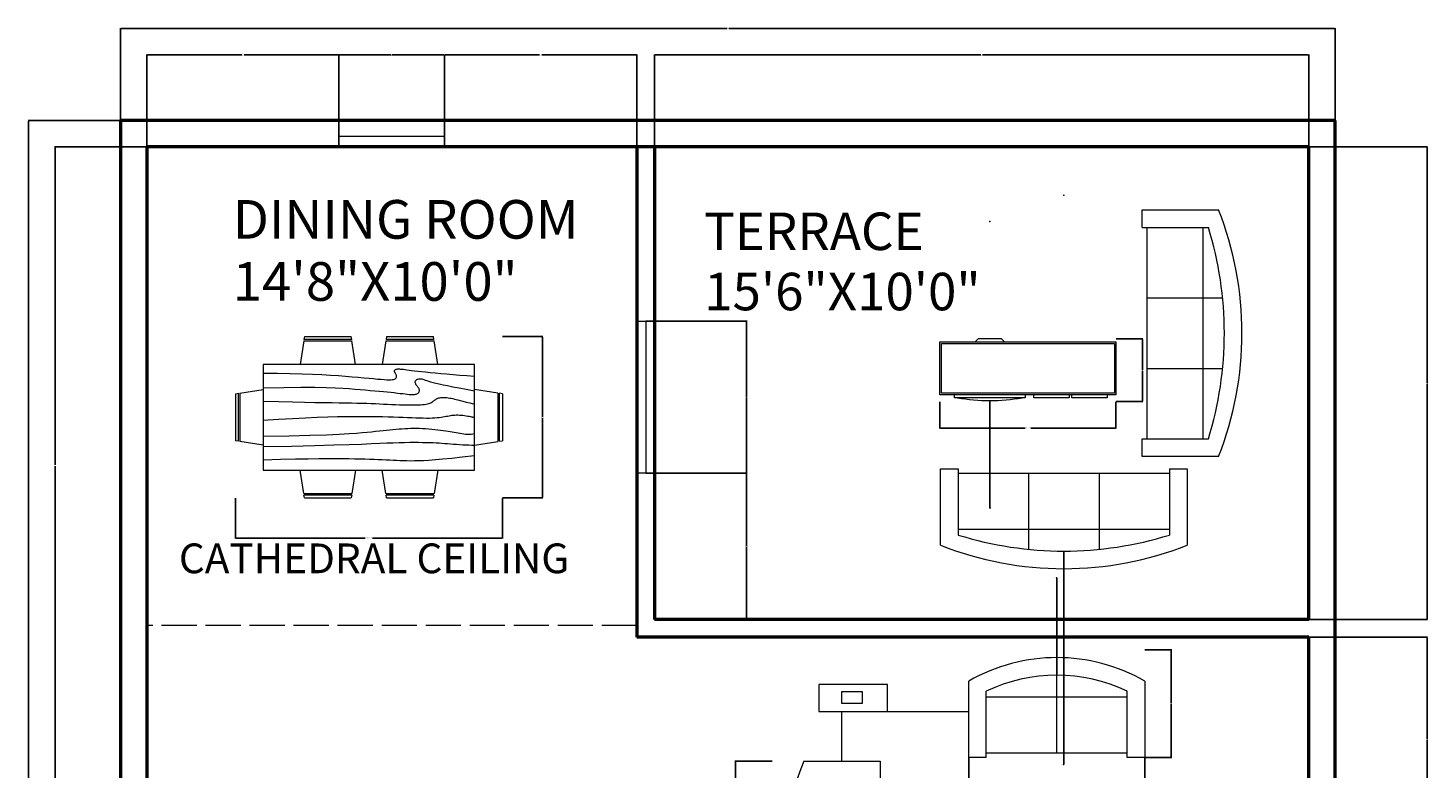
# Model space of a CAD drawing. Units: inches. Extents: x 2208 to 4689, y 1219 to 3512.
# Tile 4 of 5: x 2208 to 2685, y 1629 to 1882. Entities that reach past the tile are written whole.
import ezdxf

# ---------------------------------------------------------------- set-up
doc = ezdxf.new("R2010")
doc.units = ezdxf.units.IN
doc.linetypes.add('ACAD_ISO02W100', pattern=[15, 12, -3])
for name, color, linetype, lineweight in [('A-ANNO-DIMS', 2, 'Continuous', 18), ('A-ANNO-TEXT', 7, 'Continuous', 18), ('A-AREA-IDEN', 7, 'Continuous', 18), ('A-CLNG-OVHD', 8, 'ACAD_ISO02W100', 18), ('A-FURN', 8, 'Continuous', 18), ('A-GLAZ', 4, 'Continuous', 18), ('A-WALL', 7, 'Continuous', 50)]:
    doc.layers.add(name, color=color, linetype=linetype, lineweight=lineweight)
doc.styles.get("Standard").update_dxf_attribs({"font": 'arial.ttf'})
doc.dimstyles.get("Standard").update_dxf_attribs({"dimtxt": 0.18, "dimasz": 0.18, "dimexe": 0.18, "dimexo": 0.0625, "dimgap": 0.09, "dimtad": 0, "dimtih": 1, "dimtoh": 1, "dimdec": 4, "dimzin": 0, "dimdsep": 46, "dimtxsty": 'Standard', "dimcen": 0.09, "dimadec": 0, "dimazin": 0, "dimtfac": 1, "dimtdec": 4, "dimtofl": 0, "dimtmove": 0, "dimatfit": 3, "dimfxl": 1, "dimtolj": 1, "dimtzin": 0, "dimarcsym": 0})

# ---------------------------------------------------------------- blocks, each defined once
blk = doc.blocks.new('*U2')
for p, q in [((0, 4), (0, 0)), ((0, 2), (36, 2)), ((36, 4), (36, 0))]:
    blk.add_line(p, q)
blk = doc.blocks.new('Dining Set - 36 x 72 in.')
for p, q in [((-22.2343, 26.00059), (-23.4847, 17.99762)), ((-22.2304, 26), (-5.7608, 26)), ((-22, 27.5), (-22.1562, 26.50042)), ((-5.8416, 26.5), (-22.1534, 26.5)), ((-22, 27.5), (-6, 27.5)), ((-5.8437, 26.49966), (-6, 27.5)), ((-4.5152, 17.99762), (-5.7655, 25.99926)), ((5.7657, 26.00059), (4.5153, 17.99762)), ((5.7696, 26), (22.2392, 26)), ((6, 27.5), (5.8438, 26.50042)), ((22.1584, 26.5), (5.8466, 26.5)), ((6, 27.5), (22, 27.5)), ((22.1563, 26.49966), (22, 27.5)), ((23.4848, 17.99762), (22.2345, 25.99926)), ((36, 18), (-36, 18)), ((-36, 18), (-36, -18)), ((36, -18), (36, 18)), ((-45.5, 8), (-44.5004, 8.15617)), ((-45.5, 8), (-45.5, -8)), ((-44.5, -8.15843), (-44.5, 8.15338)), ((-44.0006, 8.23428), (-35.9976, 9.48474)), ((-44, 8.23041), (-44, -8.23915)), ((44.0006, 8.23428), (35.9976, 9.48474)), ((44, 8.23041), (44, -8.23915)), ((44.5, -8.15843), (44.5, 8.15338)), ((45.5, 8), (44.5005, 8.15617)), ((45.5, 8), (45.5, -8)), ((-44.4997, -8.15631), (-45.5, -8)), ((-35.9976, -9.48476), (-43.9993, -8.2345)), ((35.9976, -9.48476), (43.9993, -8.2345)), ((44.4997, -8.15631), (45.5, -8)), ((-36, -18), (36, -18)), ((-22.2343, -26.0006), (-23.4847, -17.99762)), ((-4.5152, -17.99762), (-5.7655, -25.99928)), ((5.7657, -26.0006), (4.5153, -17.99762)), ((23.4848, -17.99762), (22.2345, -25.99928)), ((-22.2304, -26), (-5.7608, -26)), ((-22, -27.5), (-22.1562, -26.50044)), ((-5.8416, -26.5), (-22.1534, -26.5)), ((-22, -27.5), (-6, -27.5)), ((-5.8437, -26.49967), (-6, -27.5)), ((5.7696, -26), (22.2392, -26)), ((6, -27.5), (5.8438, -26.50044)), ((22.1584, -26.5), (5.8466, -26.5)), ((6, -27.5), (22, -27.5)), ((22.1563, -26.49967), (22, -27.5))]:
    blk.add_line(p, q)
for points in [[(-36, 15), (-31.1772, 14.97754), (-26.8079, 14.91406), (-22.8538, 14.81543), (-19.276, 14.6875), (-16.0362, 14.53613), (-13.0957, 14.36718), (-10.4159, 14.18652), (-7.9583, 14), (-5.6904, 13.81315), (-3.6035, 13.63021), (-1.6954, 13.45508), (0.0365, 13.29166), (1.5945, 13.14388), (2.9811, 13.01562), (4.1988, 12.9108), (5.25, 12.83333), (6.1393, 12.78613), (6.8802, 12.76823), (7.4883, 12.77767), (7.9792, 12.8125), (8.3685, 12.87077), (8.6719, 12.95052), (8.9049, 13.0498), (9.0833, 13.16666), (9.2205, 13.29899), (9.3216, 13.44401), (9.3895, 13.59879), (9.4271, 13.76041), (9.4373, 13.92594), (9.4232, 14.09245), (9.3875, 14.257), (9.3333, 14.41666), (9.2638, 14.56917), (9.1836, 14.71484), (9.0975, 14.85465), (9.0104, 14.98958), (8.9272, 15.1206), (8.8529, 15.2487), (8.7922, 15.37483), (8.75, 15.5), (8.7305, 15.62467), (8.7344, 15.74739), (8.7617, 15.86621), (8.8125, 15.97916), (8.8867, 16.08431), (8.9844, 16.17968), (9.1055, 16.26334), (9.25, 16.33333), (9.4189, 16.38802), (9.6172, 16.42708), (9.8506, 16.45052), (10.125, 16.45833), (10.4463, 16.45052), (10.8203, 16.42708), (11.2529, 16.38802), (11.75, 16.33333), (12.3184, 16.26318), (12.9694, 16.17838), (13.7151, 16.07991), (14.5677, 15.96875), (15.5395, 15.84586), (16.6426, 15.71224), (17.8893, 15.56884), (19.2917, 15.41666), (20.859, 15.25667), (22.5879, 15.08984), (24.4721, 14.91715), (26.5052, 14.73958), (28.6809, 14.5581), (30.9929, 14.3737), (33.4347, 14.18733), (36, 14)], [(-36, 10), (-28.9766, 10.14274), (-23.1725, 10.20442), (-18.4241, 10.19775), (-14.5677, 10.13541), (-11.4399, 10.03011), (-8.877, 9.89453), (-6.7154, 9.74137), (-4.7917, 9.58333), (-2.9698, 9.43082), (-1.2246, 9.28515), (0.4415, 9.14534), (2.026, 9.01041), (3.5266, 8.87939), (4.9408, 8.7513), (6.266, 8.62516), (7.5, 8.5), (8.6411, 8.37549), (9.6914, 8.2539), (10.6538, 8.13818), (11.5312, 8.03125), (12.3267, 7.93603), (13.043, 7.85547), (13.6831, 7.79248), (14.25, 7.75), (14.7471, 7.7303), (15.1797, 7.73307), (15.5537, 7.75732), (15.875, 7.80208), (16.1494, 7.86637), (16.3828, 7.94922), (16.5811, 8.04964), (16.75, 8.16666), (16.8944, 8.29915), (17.0143, 8.44531), (17.1089, 8.60319), (17.1771, 8.77083), (17.218, 8.94629), (17.2305, 9.1276), (17.2137, 9.31282), (17.1667, 9.5), (17.0895, 9.6875), (16.987, 9.875), (16.8649, 10.0625), (16.7292, 10.25), (16.5856, 10.4375), (16.4401, 10.625), (16.2985, 10.8125), (16.1667, 11), (16.05, 11.18733), (15.9518, 11.3737), (15.8752, 11.5581), (15.8229, 11.73958), (15.798, 11.91715), (15.8034, 12.08984), (15.842, 12.25667), (15.9167, 12.41666), (16.0295, 12.56836), (16.1784, 12.70833), (16.3605, 12.83268), (16.5729, 12.9375), (16.8127, 13.01888), (17.0768, 13.07291), (17.3625, 13.0957), (17.6667, 13.08333), (17.9894, 13.03312), (18.3418, 12.94726), (18.7382, 12.82918), (19.1927, 12.68229), (19.7195, 12.51001), (20.3327, 12.31575), (21.0465, 12.10294), (21.875, 11.875), (22.8357, 11.63354), (23.959, 11.37304), (25.2786, 11.08618), (26.8282, 10.76562), (28.6414, 10.40405), (30.752, 9.99414), (33.1936, 9.52856), (36, 9)], [(-36, 5.5), (-30.7157, 5.3348), (-26.069, 5.20963), (-21.9946, 5.11767), (-18.4271, 5.05208), (-15.3009, 5.00602), (-12.5508, 4.97265), (-10.1112, 4.94515), (-7.9167, 4.91666), (-5.909, 4.88167), (-4.0586, 4.83984), (-2.3429, 4.79215), (-0.7396, 4.73958), (0.7739, 4.6831), (2.22, 4.6237), (3.6213, 4.56233), (5, 4.5), (6.373, 4.43782), (7.7344, 4.3776), (9.0723, 4.32129), (10.375, 4.27083), (11.6309, 4.22819), (12.8281, 4.19531), (13.9551, 4.17415), (15, 4.16666), (15.954, 4.17448), (16.819, 4.19791), (17.6001, 4.23698), (18.3021, 4.29166), (18.9299, 4.36198), (19.4883, 4.44791), (19.9823, 4.54948), (20.4167, 4.66666), (20.7969, 4.79899), (21.1302, 4.94401), (21.4245, 5.09879), (21.6875, 5.26041), (21.9271, 5.42594), (22.1511, 5.59245), (22.3672, 5.757), (22.5834, 5.91666), (22.8065, 6.06868), (23.0404, 6.21093), (23.2879, 6.34147), (23.5521, 6.45833), (23.8358, 6.55957), (24.142, 6.64323), (24.4735, 6.70735), (24.8334, 6.75), (25.2235, 6.76969), (25.642, 6.76692), (26.0858, 6.74267), (26.5521, 6.69791), (27.0379, 6.63362), (27.5404, 6.55078), (28.0565, 6.45036), (28.5834, 6.33333), (29.1242, 6.19987), (29.7071, 6.04687), (30.3661, 5.87044), (31.1354, 5.66666), (32.0493, 5.43164), (33.142, 5.16146), (34.4475, 4.85221), (36, 4.5)], [(-36, -1), (-30.7915, -0.6591), (-26.0195, -0.38216), (-21.6519, -0.16284), (-17.6563, 0.00521), (-14.0005, 0.12833), (-10.6523, 0.21289), (-7.5796, 0.26522), (-4.75, 0.29166), (-2.134, 0.29793), (0.2878, 0.28711), (2.5317, 0.26163), (4.6146, 0.22396), (6.5529, 0.17651), (8.3633, 0.12174), (10.0623, 0.06209), (11.6667, 0), (13.1899, -0.06201), (14.6341, -0.1211), (15.9982, -0.17432), (17.2813, -0.21875), (18.4823, -0.25147), (19.6003, -0.26953), (20.6343, -0.27002), (21.5834, -0.25), (22.4481, -0.20768), (23.2357, -0.14584), (23.9549, -0.06836), (24.6146, 0.02083), (25.2235, 0.11784), (25.7904, 0.21875), (26.3241, 0.31966), (26.8334, 0.41666), (27.3265, 0.50618), (27.8099, 0.58593), (28.2894, 0.65397), (28.7709, 0.70833), (29.2601, 0.74707), (29.763, 0.76823), (30.2855, 0.76985), (30.8334, 0.75), (31.4088, 0.70784), (31.9994, 0.64713), (32.589, 0.57275), (33.1615, 0.48958), (33.7008, 0.4025), (34.1908, 0.3164), (34.6153, 0.23616), (34.9584, 0.16666), (35.2099, 0.11165), (35.3848, 0.07031), (35.504, 0.04069), (35.5886, 0.02083), (35.6594, 0.00879), (35.7377, 0.0026), (35.8442, 0.00032), (36, 0)], [(-36, -6.5), (-27.1843, -6.31267), (-20.084, -6.1263), (-14.469, -5.9419), (-10.1094, -5.76042), (-6.7752, -5.58285), (-4.2363, -5.41016), (-2.2629, -5.24333), (-0.625, -5.08334), (0.8708, -4.93099), (2.2715, -4.78646), (3.5872, -4.64974), (4.8281, -4.52084), (6.0046, -4.39974), (7.127, -4.28646), (8.2053, -4.18099), (9.25, -4.08334), (10.2705, -3.99382), (11.2734, -3.91407), (12.2647, -3.84603), (13.25, -3.79167), (14.2354, -3.75293), (15.2266, -3.73177), (16.2295, -3.73015), (17.25, -3.75), (18.2912, -3.79248), (19.3451, -3.85547), (20.4009, -3.93604), (21.4479, -4.03125), (22.4754, -4.13819), (23.4727, -4.25391), (24.4289, -4.37549), (25.3334, -4.5), (26.1785, -4.62492), (26.9694, -4.74935), (27.7145, -4.87281), (28.4219, -4.99479), (29.1, -5.11483), (29.7572, -5.23242), (30.4016, -5.34709), (31.0417, -5.45834), (31.6837, -5.56437), (32.3262, -5.65821), (32.9658, -5.73153), (33.599, -5.77604), (34.2224, -5.78345), (34.8327, -5.74545), (35.4264, -5.65373), (36, -5.5)], [(-36, -10), (-26.4022, -9.81299), (-18.4675, -9.62891), (-11.9839, -9.45069), (-6.7396, -9.28125), (-2.5226, -9.12354), (0.8789, -8.98047), (3.6769, -8.85498), (6.0833, -8.75), (8.2767, -8.66765), (10.3021, -8.60677), (12.1712, -8.56543), (13.8958, -8.54167), (15.4876, -8.53353), (16.9583, -8.53907), (18.3197, -8.55632), (19.5834, -8.58334), (20.7616, -8.61841), (21.8685, -8.66081), (22.9188, -8.71004), (23.9271, -8.76563), (24.9081, -8.82707), (25.8763, -8.89388), (26.8465, -8.96558), (27.8334, -9.04167), (28.8474, -9.12118), (29.8828, -9.20117), (30.93, -9.27824), (31.9792, -9.34896), (33.0205, -9.40991), (34.0443, -9.45768), (35.0407, -9.48885), (36, -9.5)], [(-36, -14.5), (-30.0881, -14.33513), (-25.0332, -14.21224), (-20.7312, -14.12647), (-17.0781, -14.07292), (-13.97, -14.04671), (-11.3027, -14.04297), (-8.9724, -14.05681), (-6.875, -14.08334), (-4.9224, -14.11833), (-3.0905, -14.16016), (-1.3709, -14.20785), (0.2448, -14.26042), (1.7647, -14.3169), (3.1973, -14.3763), (4.5507, -14.43767), (5.8333, -14.5), (7.0554, -14.5621), (8.235, -14.62175), (9.3922, -14.67652), (10.5469, -14.72396), (11.7192, -14.76164), (12.929, -14.78711), (14.1965, -14.79794), (15.5417, -14.79167), (16.9933, -14.76424), (18.6152, -14.70508), (20.4804, -14.60197), (22.6615, -14.44271), (25.2312, -14.21509), (28.2624, -13.9069), (31.8277, -13.50594), (36, -13)]]:
    blk.add_lwpolyline(points)
blk = doc.blocks.new('Sofa - Roundback 7 ft.')
for p, q in [((-12.00002, -32.4421), (-12.00003, -6.5971)), ((11.99997, -32.4421), (11.99998, -6.5971)), ((-36.000027, -34), (-36.000027, -11.4696)), ((-35.999844, -13.3819), (35.9998, -13.3819)), ((35.99998, -34), (35.99998, -11.4696)), ((-36.000027, -32.4421), (35.99998, -32.4421))]:
    blk.add_line(p, q)
for points in [[(-36.000027, -34), (-42.000027, -34), (-42.000027, -8)], [(41.99998, -8), (41.99998, -34), (35.99998, -34)]]:
    blk.add_lwpolyline(points)
for centre, radius, start, end in [((0, -114.25), 114.25, 68.43141, 111.5686), ((-0.00001, -127.1968), 121.1968, 72.72033, 107.2797)]:
    blk.add_arc(centre, radius, start, end)
blk = doc.blocks.new('Sofa - Roundback Loveseat 5 ft.')
for p, q in [((0, -32.44198), (0, -5.99998)), ((-24, -33.99998), (-24, -11.46958)), ((-23.9998, -13.38178), (23.99986, -13.38178)), ((24.00004, -33.99998), (24.00004, -11.46958)), ((-24, -32.44198), (24.00004, -32.44198))]:
    blk.add_line(p, q)
for points in [[(-24, -33.99998), (-30, -33.99998), (-30, -7.99998)], [(30.00004, -7.99998), (30.00004, -33.99998), (24.00004, -33.99998)]]:
    blk.add_lwpolyline(points)
for centre, radius, start, end in [((0, -60.24998), 60.24998, 60.13715, 119.8628), ((0, -61.38438), 55.38444, 64.32083, 115.6792)]:
    blk.add_arc(centre, radius, start, end)
blk = doc.blocks.new('Entertainment Center')
for p, q in [((-4, 0), (-5, -1)), ((4, 0), (-4, 0)), ((5, -1), (4, 0)), ((-17, -19), (-17, -1)), ((-17, -1), (43, -1)), ((-16.5, -18.5), (-16.5, -1.5)), ((-16.5, -1.5), (42.5, -1.5)), ((42.5, -1.5), (42.5, -18.5)), ((43, -1), (43, -19)), ((43, -19), (-17, -19)), ((42.5, -18.5), (-16.5, -18.5)), ((-12, -20), (-12, -19)), ((12, -19), (12, -20)), ((15, -20), (15, -19)), ((27, -19), (27, -20)), ((28, -20), (28, -19)), ((40, -19), (40, -20)), ((12, -20), (-12, -20)), ((27, -20), (15, -20)), ((40, -20), (28, -20))]:
    blk.add_line(p, q)
blk.add_arc((0, 40), 61, 259.6111, 280.3889)
blk = doc.blocks.new('*D16')
at = {"layer": 'A-ANNO-DIMS', "color": 0, "lineweight": -2, "transparency": 16777216}
for p, q in [((2278.25, 1721.74), (2278.25, 1707.97)), ((2369.25, 1721.74), (2369.25, 1707.97)), ((2278.43, 1708.15), (2322.47, 1708.15)), ((2369.07, 1708.15), (2325.02, 1708.15))]:
    blk.add_line(p, q, dxfattribs=at)
at = {"layer": 'A-ANNO-DIMS', "color": 0, "transparency": 16777216}
for points in [[(2278.43, 1708.18), (2278.43, 1708.12), (2278.25, 1708.15)], [(2369.07, 1708.18), (2369.07, 1708.12), (2369.25, 1708.15)]]:
    blk.add_solid(points, dxfattribs=at)
at = {"layer": 'Defpoints', "color": 0, "transparency": 16777216}
for p in [(2278.25, 1721.8), (2369.25, 1721.8), (2369.25, 1708.15)]:
    blk.add_point(p, dxfattribs=at)
at = {"layer": 'A-ANNO-DIMS', "color": 0, "transparency": 16777216, "insert": (2323.75, 1708.15), "char_height": 0.18, "attachment_point": 5}
blk.add_mtext('\\A1;DINING SET 91 TYP.', dxfattribs=at)
blk = doc.blocks.new('*D17')
at = {"layer": 'A-ANNO-DIMS', "color": 0, "lineweight": -2, "transparency": 16777216}
for p, q in [((2369.31, 1776.8), (2383.08, 1776.8)), ((2382.9, 1776.62), (2382.9, 1749.48)), ((2382.9, 1721.98), (2382.9, 1749.12)), ((2369.31, 1721.8), (2383.08, 1721.8))]:
    blk.add_line(p, q, dxfattribs=at)
at = {"layer": 'A-ANNO-DIMS', "color": 0, "transparency": 16777216}
for points in [[(2382.87, 1776.62), (2382.93, 1776.62), (2382.9, 1776.8)], [(2382.87, 1721.98), (2382.93, 1721.98), (2382.9, 1721.8)]]:
    blk.add_solid(points, dxfattribs=at)
at = {"layer": 'Defpoints', "color": 0, "transparency": 16777216}
for p in [(2369.25, 1776.8), (2382.9, 1776.8), (2369.25, 1721.8)]:
    blk.add_point(p, dxfattribs=at)
at = {"layer": 'A-ANNO-DIMS', "color": 0, "transparency": 16777216, "insert": (2382.9, 1749.3), "char_height": 0.18, "attachment_point": 5}
blk.add_mtext('\\A1;55 TYP.', dxfattribs=at)
blk = doc.blocks.new('*D18')
at = {"layer": 'A-ANNO-DIMS', "color": 0, "lineweight": -2, "transparency": 16777216}
for p, q in [((2528.21, 1633.35), (2528.21, 1624.23)), ((2588.21, 1633.35), (2588.21, 1624.23)), ((2528.39, 1624.41), (2556.98, 1624.41)), ((2588.03, 1624.41), (2559.43, 1624.41))]:
    blk.add_line(p, q, dxfattribs=at)
at = {"layer": 'A-ANNO-DIMS', "color": 0, "transparency": 16777216}
for points in [[(2528.39, 1624.44), (2528.39, 1624.38), (2528.21, 1624.41)], [(2588.03, 1624.44), (2588.03, 1624.38), (2588.21, 1624.41)]]:
    blk.add_solid(points, dxfattribs=at)
at = {"layer": 'Defpoints', "color": 0, "transparency": 16777216}
for p in [(2528.21, 1633.41), (2588.21, 1633.41), (2588.21, 1624.41)]:
    blk.add_point(p, dxfattribs=at)
at = {"layer": 'A-ANNO-DIMS', "color": 0, "transparency": 16777216, "insert": (2558.21, 1624.41), "char_height": 0.18, "attachment_point": 5}
blk.add_mtext('\\A1;LOVESEAT 60 TYP.', dxfattribs=at)
blk = doc.blocks.new('*D19')
at = {"layer": 'A-ANNO-DIMS', "color": 0, "lineweight": -2, "transparency": 16777216}
for p, q in [((2588.27, 1670.08), (2597.39, 1670.08)), ((2597.21, 1669.9), (2597.21, 1651.92)), ((2597.21, 1633.59), (2597.21, 1651.56)), ((2588.27, 1633.41), (2597.39, 1633.41))]:
    blk.add_line(p, q, dxfattribs=at)
at = {"layer": 'A-ANNO-DIMS', "color": 0, "transparency": 16777216}
for points in [[(2597.18, 1669.9), (2597.24, 1669.9), (2597.21, 1670.08)], [(2597.18, 1633.59), (2597.24, 1633.59), (2597.21, 1633.41)]]:
    blk.add_solid(points, dxfattribs=at)
at = {"layer": 'Defpoints', "color": 0, "transparency": 16777216}
for p in [(2588.21, 1670.08), (2597.21, 1670.08), (2588.21, 1633.41)]:
    blk.add_point(p, dxfattribs=at)
at = {"layer": 'A-ANNO-DIMS', "color": 0, "transparency": 16777216, "insert": (2597.21, 1651.74), "char_height": 0.18, "attachment_point": 5}
blk.add_mtext('\\A1;37 TYP.', dxfattribs=at)
blk = doc.blocks.new('*D20')
at = {"layer": 'A-ANNO-DIMS', "color": 0, "lineweight": -2, "transparency": 16777216}
for p, q in [((2461.24, 1632.1), (2448.52, 1632.1)), ((2448.7, 1631.92), (2448.7, 1590.28)), ((2448.7, 1548.28), (2448.7, 1589.91)), ((2461.24, 1548.1), (2448.52, 1548.1))]:
    blk.add_line(p, q, dxfattribs=at)
at = {"layer": 'A-ANNO-DIMS', "color": 0, "transparency": 16777216}
for points in [[(2448.67, 1631.92), (2448.73, 1631.92), (2448.7, 1632.1)], [(2448.67, 1548.28), (2448.73, 1548.28), (2448.7, 1548.1)]]:
    blk.add_solid(points, dxfattribs=at)
at = {"layer": 'Defpoints', "color": 0, "transparency": 16777216}
for p in [(2448.7, 1632.1), (2461.3, 1632.1), (2461.3, 1548.1)]:
    blk.add_point(p, dxfattribs=at)
at = {"layer": 'A-ANNO-DIMS', "color": 0, "transparency": 16777216, "insert": (2448.7, 1590.1), "char_height": 0.18, "attachment_point": 5}
blk.add_mtext('\\A1;SOFA 84 TYP.', dxfattribs=at)
blk = doc.blocks.new('*D32')
at = {"layer": 'A-ANNO-DIMS', "color": 0, "lineweight": -2, "transparency": 16777216}
for p, q in [((2518.4, 1754.56), (2518.4, 1745.44)), ((2578.4, 1754.56), (2578.4, 1745.44)), ((2518.58, 1745.62), (2547.43, 1745.62)), ((2578.22, 1745.62), (2549.38, 1745.62))]:
    blk.add_line(p, q, dxfattribs=at)
at = {"layer": 'A-ANNO-DIMS', "color": 0, "transparency": 16777216}
for points in [[(2518.58, 1745.65), (2518.58, 1745.59), (2518.4, 1745.62)], [(2578.22, 1745.65), (2578.22, 1745.59), (2578.4, 1745.62)]]:
    blk.add_solid(points, dxfattribs=at)
at = {"layer": 'Defpoints', "color": 0, "transparency": 16777216}
for p in [(2518.4, 1754.62), (2578.4, 1754.62), (2578.4, 1745.62)]:
    blk.add_point(p, dxfattribs=at)
at = {"layer": 'A-ANNO-DIMS', "color": 0, "transparency": 16777216, "insert": (2548.4, 1745.62), "char_height": 0.18, "attachment_point": 5}
blk.add_mtext('\\A1;MEDIA UNIT 60', dxfattribs=at)
blk = doc.blocks.new('*D33')
at = {"layer": 'A-ANNO-DIMS', "color": 0, "lineweight": -2, "transparency": 16777216}
for p, q in [((2578.46, 1775.95), (2587.58, 1775.95)), ((2587.4, 1775.77), (2587.4, 1765.47)), ((2587.4, 1754.8), (2587.4, 1765.11)), ((2578.46, 1754.62), (2587.58, 1754.62))]:
    blk.add_line(p, q, dxfattribs=at)
at = {"layer": 'A-ANNO-DIMS', "color": 0, "transparency": 16777216}
for points in [[(2587.37, 1775.77), (2587.43, 1775.77), (2587.4, 1775.95)], [(2587.37, 1754.8), (2587.43, 1754.8), (2587.4, 1754.62)]]:
    blk.add_solid(points, dxfattribs=at)
at = {"layer": 'Defpoints', "color": 0, "transparency": 16777216}
for p in [(2578.4, 1775.95), (2587.4, 1775.95), (2578.4, 1754.62)]:
    blk.add_point(p, dxfattribs=at)
at = {"layer": 'A-ANNO-DIMS', "color": 0, "transparency": 16777216, "insert": (2587.4, 1765.29), "char_height": 0.18, "attachment_point": 5}
blk.add_mtext('\\A1;21', dxfattribs=at)
blk = doc.blocks.new('*D34')
at = {"layer": 'A-ANNO-DIMS', "color": 0, "lineweight": -2, "transparency": 16777216}
for p, q in [((2239.1, 1850.42), (2239.1, 1881.89)), ((2239.28, 1881.71), (2445.81, 1881.71)), ((2652.92, 1881.71), (2446.39, 1881.71)), ((2653.1, 1850.42), (2653.1, 1881.89))]:
    blk.add_line(p, q, dxfattribs=at)
at = {"layer": 'A-ANNO-DIMS', "color": 0, "transparency": 16777216}
for points in [[(2239.28, 1881.74), (2239.28, 1881.68), (2239.1, 1881.71)], [(2652.92, 1881.74), (2652.92, 1881.68), (2653.1, 1881.71)]]:
    blk.add_solid(points, dxfattribs=at)
at = {"layer": 'Defpoints', "color": 0, "transparency": 16777216}
for p in [(2653.1, 1881.71), (2239.1, 1850.36), (2653.1, 1850.36)]:
    blk.add_point(p, dxfattribs=at)
at = {"layer": 'A-ANNO-DIMS', "color": 0, "transparency": 16777216, "insert": (2446.1, 1881.71), "char_height": 0.18, "attachment_point": 5}
blk.add_mtext('\\A1;414', dxfattribs=at)
blk = doc.blocks.new('*D35')
at = {"layer": 'A-ANNO-DIMS', "color": 0, "lineweight": -2, "transparency": 16777216}
for p, q in [((2239.04, 1850.36), (2207.57, 1850.36)), ((2207.75, 1850.18), (2207.75, 1550.54)), ((2207.75, 1250.54), (2207.75, 1550.17)), ((2239.04, 1250.36), (2207.57, 1250.36))]:
    blk.add_line(p, q, dxfattribs=at)
at = {"layer": 'A-ANNO-DIMS', "color": 0, "transparency": 16777216}
for points in [[(2207.72, 1850.18), (2207.78, 1850.18), (2207.75, 1850.36)], [(2207.72, 1250.54), (2207.78, 1250.54), (2207.75, 1250.36)]]:
    blk.add_solid(points, dxfattribs=at)
at = {"layer": 'Defpoints', "color": 0, "transparency": 16777216}
for p in [(2207.75, 1850.36), (2239.1, 1850.36), (2239.1, 1250.36)]:
    blk.add_point(p, dxfattribs=at)
at = {"layer": 'A-ANNO-DIMS', "color": 0, "transparency": 16777216, "insert": (2207.75, 1550.36), "char_height": 0.18, "attachment_point": 5}
blk.add_mtext('\\A1;600', dxfattribs=at)
blk = doc.blocks.new('*D36')
at = {"layer": 'A-ANNO-DIMS', "color": 0, "lineweight": -2, "transparency": 16777216}
for p, q in [((2248.1, 1841.42), (2248.1, 1872.89)), ((2248.28, 1872.71), (2280.43, 1872.71)), ((2313.33, 1872.71), (2281.18, 1872.71)), ((2313.51, 1841.42), (2313.51, 1872.89))]:
    blk.add_line(p, q, dxfattribs=at)
at = {"layer": 'A-ANNO-DIMS', "color": 0, "transparency": 16777216}
for points in [[(2248.28, 1872.74), (2248.28, 1872.68), (2248.1, 1872.71)], [(2313.33, 1872.74), (2313.33, 1872.68), (2313.51, 1872.71)]]:
    blk.add_solid(points, dxfattribs=at)
at = {"layer": 'Defpoints', "color": 0, "transparency": 16777216}
for p in [(2313.51, 1872.71), (2248.1, 1841.36), (2313.51, 1841.36)]:
    blk.add_point(p, dxfattribs=at)
at = {"layer": 'A-ANNO-DIMS', "color": 0, "transparency": 16777216, "insert": (2280.8, 1872.71), "char_height": 0.18, "attachment_point": 5}
blk.add_mtext('\\A1;65.41', dxfattribs=at)
blk = doc.blocks.new('*D37')
at = {"layer": 'A-ANNO-DIMS', "color": 0, "lineweight": -2, "transparency": 16777216}
for p, q in [((2313.51, 1841.42), (2313.51, 1872.89)), ((2313.69, 1872.71), (2331.29, 1872.71)), ((2349.33, 1872.71), (2331.73, 1872.71)), ((2349.51, 1841.42), (2349.51, 1872.89))]:
    blk.add_line(p, q, dxfattribs=at)
at = {"layer": 'A-ANNO-DIMS', "color": 0, "transparency": 16777216}
for points in [[(2313.69, 1872.74), (2313.69, 1872.68), (2313.51, 1872.71)], [(2349.33, 1872.74), (2349.33, 1872.68), (2349.51, 1872.71)]]:
    blk.add_solid(points, dxfattribs=at)
at = {"layer": 'Defpoints', "color": 0, "transparency": 16777216}
for p in [(2349.51, 1872.71), (2313.51, 1841.36), (2349.51, 1841.36)]:
    blk.add_point(p, dxfattribs=at)
at = {"layer": 'A-ANNO-DIMS', "color": 0, "transparency": 16777216, "insert": (2331.51, 1872.71), "char_height": 0.18, "attachment_point": 5}
blk.add_mtext('\\A1;36', dxfattribs=at)
blk = doc.blocks.new('*D38')
at = {"layer": 'A-ANNO-DIMS', "color": 0, "lineweight": -2, "transparency": 16777216}
for p, q in [((2349.51, 1841.42), (2349.51, 1872.89)), ((2349.69, 1872.71), (2381.91, 1872.71)), ((2414.92, 1872.71), (2382.7, 1872.71)), ((2415.1, 1841.42), (2415.1, 1872.89))]:
    blk.add_line(p, q, dxfattribs=at)
at = {"layer": 'A-ANNO-DIMS', "color": 0, "transparency": 16777216}
for points in [[(2349.69, 1872.74), (2349.69, 1872.68), (2349.51, 1872.71)], [(2414.92, 1872.74), (2414.92, 1872.68), (2415.1, 1872.71)]]:
    blk.add_solid(points, dxfattribs=at)
at = {"layer": 'Defpoints', "color": 0, "transparency": 16777216}
for p in [(2415.1, 1872.71), (2349.51, 1841.36), (2415.1, 1841.36)]:
    blk.add_point(p, dxfattribs=at)
at = {"layer": 'A-ANNO-DIMS', "color": 0, "transparency": 16777216, "insert": (2382.3, 1872.71), "char_height": 0.18, "attachment_point": 5}
blk.add_mtext('\\A1;65.59', dxfattribs=at)
blk = doc.blocks.new('*D39')
at = {"layer": 'A-ANNO-DIMS', "color": 0, "lineweight": -2, "transparency": 16777216}
for p, q in [((2421.1, 1841.42), (2421.1, 1872.89)), ((2421.28, 1872.71), (2532.31, 1872.71)), ((2643.92, 1872.71), (2532.89, 1872.71)), ((2644.1, 1841.42), (2644.1, 1872.89))]:
    blk.add_line(p, q, dxfattribs=at)
at = {"layer": 'A-ANNO-DIMS', "color": 0, "transparency": 16777216}
for points in [[(2421.28, 1872.74), (2421.28, 1872.68), (2421.1, 1872.71)], [(2643.92, 1872.74), (2643.92, 1872.68), (2644.1, 1872.71)]]:
    blk.add_solid(points, dxfattribs=at)
at = {"layer": 'Defpoints', "color": 0, "transparency": 16777216}
for p in [(2644.1, 1872.71), (2421.1, 1841.36), (2644.1, 1841.36)]:
    blk.add_point(p, dxfattribs=at)
at = {"layer": 'A-ANNO-DIMS', "color": 0, "transparency": 16777216, "insert": (2532.6, 1872.71), "char_height": 0.18, "attachment_point": 5}
blk.add_mtext('\\A1;223', dxfattribs=at)
blk = doc.blocks.new('*D46')
at = {"layer": 'A-ANNO-DIMS', "color": 0, "lineweight": -2, "transparency": 16777216}
for p, q in [((2248.04, 1841.36), (2216.57, 1841.36)), ((2216.75, 1841.18), (2216.75, 1733.03)), ((2216.75, 1624.53), (2216.75, 1732.67)), ((2248.04, 1624.35), (2216.57, 1624.35))]:
    blk.add_line(p, q, dxfattribs=at)
at = {"layer": 'A-ANNO-DIMS', "color": 0, "transparency": 16777216}
for points in [[(2216.72, 1841.18), (2216.78, 1841.18), (2216.75, 1841.36)], [(2216.72, 1624.53), (2216.78, 1624.53), (2216.75, 1624.35)]]:
    blk.add_solid(points, dxfattribs=at)
at = {"layer": 'Defpoints', "color": 0, "transparency": 16777216}
for p in [(2216.75, 1841.36), (2248.1, 1841.36), (2248.1, 1624.35)]:
    blk.add_point(p, dxfattribs=at)
at = {"layer": 'A-ANNO-DIMS', "color": 0, "transparency": 16777216, "insert": (2216.75, 1732.85), "char_height": 0.18, "attachment_point": 5}
blk.add_mtext('\\A1;217', dxfattribs=at)
blk = doc.blocks.new('*D63')
at = {"layer": 'A-ANNO-DIMS', "color": 0, "lineweight": -2, "transparency": 16777216}
for p, q in [((2644.16, 1674.36), (2684.63, 1674.36)), ((2684.45, 1674.18), (2684.45, 1639.78)), ((2684.45, 1605.03), (2684.45, 1639.42)), ((2653.16, 1604.85), (2684.63, 1604.85))]:
    blk.add_line(p, q, dxfattribs=at)
at = {"layer": 'A-ANNO-DIMS', "color": 0, "transparency": 16777216}
for points in [[(2684.42, 1674.18), (2684.48, 1674.18), (2684.45, 1674.36)], [(2684.42, 1605.03), (2684.48, 1605.03), (2684.45, 1604.85)]]:
    blk.add_solid(points, dxfattribs=at)
at = {"layer": 'Defpoints', "color": 0, "transparency": 16777216}
for p in [(2644.1, 1674.36), (2684.45, 1674.36), (2653.1, 1604.85)]:
    blk.add_point(p, dxfattribs=at)
at = {"layer": 'A-ANNO-DIMS', "color": 0, "transparency": 16777216, "insert": (2684.45, 1639.6), "char_height": 0.18, "attachment_point": 5}
blk.add_mtext('\\A1;69.51', dxfattribs=at)
blk = doc.blocks.new('*D64')
at = {"layer": 'A-ANNO-DIMS', "color": 0, "lineweight": -2, "transparency": 16777216}
for p, q in [((2644.16, 1841.36), (2684.63, 1841.36)), ((2684.45, 1841.18), (2684.45, 1761.04)), ((2684.45, 1680.54), (2684.45, 1760.67)), ((2644.16, 1680.36), (2684.63, 1680.36))]:
    blk.add_line(p, q, dxfattribs=at)
at = {"layer": 'A-ANNO-DIMS', "color": 0, "transparency": 16777216}
for points in [[(2684.42, 1841.18), (2684.48, 1841.18), (2684.45, 1841.36)], [(2684.42, 1680.54), (2684.48, 1680.54), (2684.45, 1680.36)]]:
    blk.add_solid(points, dxfattribs=at)
at = {"layer": 'Defpoints', "color": 0, "transparency": 16777216}
for p in [(2644.1, 1841.36), (2684.45, 1841.36), (2644.1, 1680.36)]:
    blk.add_point(p, dxfattribs=at)
at = {"layer": 'A-ANNO-DIMS', "color": 0, "transparency": 16777216, "insert": (2684.45, 1760.86), "char_height": 0.18, "attachment_point": 5}
blk.add_mtext('\\A1;161', dxfattribs=at)
blk = doc.blocks.new('*D65')
at = {"layer": 'A-ANNO-DIMS', "color": 0, "lineweight": -2, "transparency": 16777216}
for p, q in [((2421.16, 1782.02), (2452.63, 1782.02)), ((2452.45, 1781.84), (2452.45, 1756.34)), ((2452.45, 1730.48), (2452.45, 1755.98)), ((2421.16, 1730.3), (2452.63, 1730.3))]:
    blk.add_line(p, q, dxfattribs=at)
at = {"layer": 'A-ANNO-DIMS', "color": 0, "transparency": 16777216}
for points in [[(2452.42, 1781.84), (2452.48, 1781.84), (2452.45, 1782.02)], [(2452.42, 1730.48), (2452.48, 1730.48), (2452.45, 1730.3)]]:
    blk.add_solid(points, dxfattribs=at)
at = {"layer": 'Defpoints', "color": 0, "transparency": 16777216}
for p in [(2421.1, 1782.02), (2421.1, 1730.3), (2452.45, 1730.3)]:
    blk.add_point(p, dxfattribs=at)
at = {"layer": 'A-ANNO-DIMS', "color": 0, "transparency": 16777216, "insert": (2452.45, 1756.16), "char_height": 0.18, "attachment_point": 5}
blk.add_mtext('\\A1;51.72', dxfattribs=at)
blk = doc.blocks.new('*D66')
at = {"layer": 'A-ANNO-DIMS', "color": 0, "lineweight": -2, "transparency": 16777216}
for p, q in [((2421.16, 1730.3), (2452.63, 1730.3)), ((2452.45, 1730.12), (2452.45, 1705.51)), ((2452.45, 1680.54), (2452.45, 1705.14)), ((2421.16, 1680.36), (2452.63, 1680.36))]:
    blk.add_line(p, q, dxfattribs=at)
at = {"layer": 'A-ANNO-DIMS', "color": 0, "transparency": 16777216}
for points in [[(2452.42, 1730.12), (2452.48, 1730.12), (2452.45, 1730.3)], [(2452.42, 1680.54), (2452.48, 1680.54), (2452.45, 1680.36)]]:
    blk.add_solid(points, dxfattribs=at)
at = {"layer": 'Defpoints', "color": 0, "transparency": 16777216}
for p in [(2421.1, 1730.3), (2421.1, 1680.36), (2452.45, 1680.36)]:
    blk.add_point(p, dxfattribs=at)
at = {"layer": 'A-ANNO-DIMS', "color": 0, "transparency": 16777216, "insert": (2452.45, 1705.33), "char_height": 0.18, "attachment_point": 5}
blk.add_mtext('\\A1;49.94', dxfattribs=at)
blk = doc.blocks.new('*D76')
at = {"layer": 'A-ANNO-DIMS', "color": 0, "lineweight": -2, "transparency": 16777216}
for p, q in [((2560.54, 1824.9), (2560.72, 1824.9)), ((2560.63, 1824.81), (2560.63, 1824.99)), ((2560.63, 1630.99), (2560.63, 1703.53)), ((2560.45, 1630.99), (2560.63, 1630.99))]:
    blk.add_line(p, q, dxfattribs=at)
at = {"layer": 'A-ANNO-DIMS', "color": 0, "transparency": 16777216}
blk.add_solid([(2560.6, 1703.53), (2560.66, 1703.53), (2560.63, 1703.71)], dxfattribs=at)
at = {"layer": 'Defpoints', "color": 0, "transparency": 16777216}
for p in [(2560.63, 1824.9), (2560.63, 1703.71)]:
    blk.add_point(p, dxfattribs=at)
at = {"layer": 'A-ANNO-DIMS', "color": 0, "transparency": 16777216, "insert": (2559.77, 1630.99), "char_height": 0.18, "attachment_point": 5}
blk.add_mtext('\\A1;3X R121.2', dxfattribs=at)
blk = doc.blocks.new('*D78')
at = {"layer": 'A-ANNO-DIMS', "color": 0, "lineweight": -2, "transparency": 16777216}
for p, q in [((2535.31, 1815.95), (2535.49, 1815.95)), ((2535.4, 1815.86), (2535.4, 1816.04)), ((2535.4, 1718.35), (2535.4, 1754.77)), ((2535.58, 1718.35), (2535.4, 1718.35))]:
    blk.add_line(p, q, dxfattribs=at)
at = {"layer": 'A-ANNO-DIMS', "color": 0, "transparency": 16777216}
blk.add_solid([(2535.43, 1754.77), (2535.37, 1754.77), (2535.4, 1754.95)], dxfattribs=at)
at = {"layer": 'Defpoints', "color": 0, "transparency": 16777216}
for p in [(2535.4, 1815.95), (2535.4, 1754.95)]:
    blk.add_point(p, dxfattribs=at)
at = {"layer": 'A-ANNO-DIMS', "color": 0, "transparency": 16777216, "insert": (2535.87, 1718.35), "char_height": 0.18, "attachment_point": 5}
blk.add_mtext('\\A1;R61', dxfattribs=at)
blk = doc.blocks.new('*D80')
at = {"layer": 'A-ANNO-DIMS', "color": 0, "lineweight": -2, "transparency": 16777216}
for p, q in [((2558.02, 1694.64), (2558.2, 1694.64)), ((2558.2, 1694.64), (2558.2, 1661.59)), ((2558.12, 1606.03), (2558.3, 1606.03)), ((2558.21, 1605.94), (2558.21, 1606.12))]:
    blk.add_line(p, q, dxfattribs=at)
at = {"layer": 'A-ANNO-DIMS', "color": 0, "transparency": 16777216}
blk.add_solid([(2558.23, 1661.59), (2558.17, 1661.59), (2558.2, 1661.41)], dxfattribs=at)
at = {"layer": 'Defpoints', "color": 0, "transparency": 16777216}
for p in [(2558.2, 1661.41), (2558.21, 1606.03)]:
    blk.add_point(p, dxfattribs=at)
at = {"layer": 'A-ANNO-DIMS', "color": 0, "transparency": 16777216, "insert": (2557.35, 1694.64), "char_height": 0.18, "attachment_point": 5}
blk.add_mtext('\\A1;3X R55.38', dxfattribs=at)

msp = doc.modelspace()

# ---------------------------------------------------------------- linework, layer by layer
at = {"layer": 'A-CLNG-OVHD'}
msp.add_line((2415.0983, 1678.3962), (2248.0983, 1678.3962), dxfattribs=at)
at = {"layer": 'A-FURN'}
for p, q in [((2500.4791, 1658.2144), (2477.083, 1658.2144)), ((2477.083, 1658.2144), (2477.083, 1649.07)), ((2500.4791, 1649.07), (2500.4791, 1658.2144)), ((2477.083, 1649.07), (2484.9651, 1649.07)), ((2484.9651, 1632.0963), (2484.9651, 1649.07)), ((2484.9651, 1649.07), (2528.2051, 1649.07))]:
    msp.add_line(p, q, dxfattribs=at)
msp.add_lwpolyline([(2484.8994, 1655.8272), (2491.8503, 1655.8272), (2491.8503, 1651.8141), (2484.8994, 1651.8141)], close=True, dxfattribs=at)
at = {"layer": 'A-GLAZ'}
for p, q in [((2313.5109, 1847.0092), (2313.5109, 1850.3551)), ((2349.5109, 1847.0092), (2349.5109, 1850.3551)), ((2349.5109, 1850.3551), (2349.5109, 1841.3551)), ((2313.5109, 1843.0092), (2313.5109, 1841.3551)), ((2415.0983, 1782.0203), (2421.0983, 1782.0203)), ((2421.0983, 1782.0203), (2418.0983, 1782.0203)), ((2418.0983, 1782.0203), (2418.0983, 1730.2979)), ((2421.0983, 1730.2979), (2415.0983, 1730.2979)), ((2418.0983, 1730.2979), (2421.0983, 1730.2979))]:
    msp.add_line(p, q, dxfattribs=at)
at = {"layer": 'A-WALL'}
for p, q in [((2653.0983, 1850.3551), (2239.0983, 1850.3551)), ((2239.0983, 1850.3551), (2239.0983, 1250.3551)), ((2653.0983, 1378.3551), (2653.0983, 1850.3551)), ((2248.0983, 1841.3551), (2248.0983, 1450.3551)), ((2644.0983, 1841.3551), (2248.0983, 1841.3551)), ((2415.0983, 1841.3551), (2415.0983, 1674.3551)), ((2421.0983, 1841.3551), (2421.0983, 1680.3551)), ((2644.0983, 1680.3551), (2644.0983, 1841.3551)), ((2644.0983, 1680.3551), (2421.0983, 1680.3551)), ((2644.0983, 1674.3551), (2415.0983, 1674.3551)), ((2644.0983, 1519.6482), (2644.0983, 1674.3551))]:
    msp.add_line(p, q, dxfattribs=at)

# ---------------------------------------------------------------- block references
at = {"layer": 'A-FURN'}
for p, rotation in [((2621.3508, 1777.9338), 270), ((2560.625, 1697.7082), 180), ((2463.9651, 1590.0963), 90)]:
    msp.add_blockref('Sofa - Roundback 7 ft.', p, dxfattribs=dict(at, rotation=rotation))
for name, p in [('Dining Set - 36 x 72 in.', (2323.7462, 1749.2992)), ('Entertainment Center', (2535.4016, 1775.9522)), ('Sofa - Roundback Loveseat 5 ft.', (2558.2051, 1667.4095))]:
    msp.add_blockref(name, p, dxfattribs=at)
at = {"layer": 'A-GLAZ'}
msp.add_blockref('*U2', (2313.5109, 1843.0092), dxfattribs=at)

# ---------------------------------------------------------------- texts
at = {"layer": 'A-ANNO-TEXT'}
msp.add_text('CATHEDRAL CEILING    ', height=10.129564, dxfattribs=at).set_placement((2258.9808, 1696.1634))
at = {"layer": 'A-AREA-IDEN'}
for s, height, p in [('DINING ROOM', 13.165315, (2277.3188, 1810.1189)), ('TERRACE', 12.7781, (2438.013, 1806.2502)), ('14\'8"X10\'0"', 13.165315, (2277.3188, 1788.97)), ('15\'6"X10\'0"', 12.778097, (2438.013, 1785.7233))]:
    msp.add_text(s, height=height, dxfattribs=at).set_placement(p)

# ---------------------------------------------------------------- dimensions: what is measured, and where the dimension line sits
at = {"layer": 'A-ANNO-DIMS'}
for base, p1, p2, override, picture, middle in [((2653.0983, 1881.7051), (2239.0983, 1850.3551), (2653.0983, 1850.3551), {"dimdec": 0, "dimlfac": 1, "dimrnd": 0, "dimzin": 0, "dimdsep": 46, "dimlunit": 2}, '*D34', (2446.0983, 1881.7051)), ((2313.5109, 1872.7051), (2248.0983, 1841.3551), (2313.5109, 1841.3551), {"dimdec": 2, "dimlfac": 1, "dimrnd": 0, "dimzin": 0, "dimdsep": 46, "dimlunit": 2}, '*D36', (2280.8046, 1872.7051)), ((2349.5109, 1872.7051), (2313.5109, 1841.3551), (2349.5109, 1841.3551), {"dimdec": 0, "dimlfac": 1, "dimrnd": 0, "dimzin": 0, "dimdsep": 46, "dimlunit": 2}, '*D37', (2331.5109, 1872.7051)), ((2415.0983, 1872.7051), (2349.5109, 1841.3551), (2415.0983, 1841.3551), {"dimdec": 2, "dimlfac": 1, "dimrnd": 0, "dimzin": 0, "dimdsep": 46, "dimlunit": 2}, '*D38', (2382.3046, 1872.7051)), ((2644.0983, 1872.7051), (2421.0983, 1841.3551), (2644.0983, 1841.3551), {"dimdec": 0, "dimlfac": 1, "dimrnd": 0, "dimzin": 0, "dimdsep": 46, "dimlunit": 2}, '*D39', (2532.5983, 1872.7051))]:
    dim = msp.add_linear_dim(base=base, p1=p1, p2=p2, dimstyle='Standard', override=override, dxfattribs=at)
    dim.commit()
    dim.dimension.update_dxf_attribs({"geometry": picture, "text_midpoint": middle})
for base, p1, p2, angle, override, picture, middle in [((2207.7483, 1850.3551), (2239.0983, 1250.3551), (2239.0983, 1850.3551), 90, {"dimdec": 0, "dimlfac": 1, "dimrnd": 0, "dimzin": 0, "dimdsep": 46, "dimlunit": 2}, '*D35', (2207.7483, 1550.3551)), ((2216.7483, 1841.3551), (2248.0983, 1624.3486), (2248.0983, 1841.3551), 90, {"dimdec": 0, "dimlfac": 1, "dimrnd": 0, "dimzin": 0, "dimdsep": 46, "dimlunit": 2}, '*D46', (2216.7483, 1732.8518)), ((2684.4483, 1841.3551), (2644.0983, 1680.3551), (2644.0983, 1841.3551), 90, {"dimdec": 0, "dimlfac": 1, "dimrnd": 0, "dimzin": 0, "dimdsep": 46, "dimlunit": 2}, '*D64', (2684.4483, 1760.8551)), ((2452.4483, 1730.2979), (2421.0983, 1782.0203), (2421.0983, 1730.2979), 270, {"dimdec": 2, "dimlfac": 1, "dimrnd": 0, "dimzin": 0, "dimdsep": 46, "dimlunit": 2}, '*D65', (2452.4483, 1756.1591)), ((2587.4016, 1775.9522), (2578.4016, 1754.6188), (2578.4016, 1775.9522), 90, {"dimdec": 0, "dimlfac": 1, "dimrnd": 0, "dimzin": 0, "dimdsep": 46, "dimlunit": 2}, '*D33', (2587.4016, 1765.2855)), ((2452.4483, 1680.3551), (2421.0983, 1730.2979), (2421.0983, 1680.3551), 270, {"dimdec": 2, "dimlfac": 1, "dimrnd": 0, "dimzin": 0, "dimdsep": 46, "dimlunit": 2}, '*D66', (2452.4483, 1705.3265)), ((2684.4483, 1674.3551), (2653.0983, 1604.8466), (2644.0983, 1674.3551), 90, {"dimdec": 2, "dimlfac": 1, "dimrnd": 0, "dimzin": 0, "dimdsep": 46, "dimlunit": 2}, '*D63', (2684.4483, 1639.6008))]:
    dim = msp.add_linear_dim(base=base, p1=p1, p2=p2, angle=angle, dimstyle='Standard', override=override, dxfattribs=at)
    dim.commit()
    dim.dimension.update_dxf_attribs({"geometry": picture, "text_midpoint": middle})
for center, mpoint, override, picture, middle in [((2560.625, 1824.905), (2560.625, 1703.7082), {"dimdec": 1, "dimlfac": 1, "dimrnd": 0, "dimzin": 0, "dimdsep": 46, "dimlunit": 2}, '*D76', (2559.7728, 1630.9901)), ((2558.2051, 1606.0251), (2558.205, 1661.4095), {"dimdec": 2, "dimlfac": 1, "dimrnd": 0, "dimzin": 0, "dimdsep": 46, "dimlunit": 2}, '*D80', (2557.3516, 1694.6402))]:
    dim = msp.add_radius_dim(center=center, mpoint=mpoint, text='3X <>', dimstyle='Standard', override=override, dxfattribs=at)
    dim.commit()
    dim.dimension.update_dxf_attribs({"geometry": picture, "text_midpoint": middle, "dimtype": 164})
dim = msp.add_radius_dim(center=(2535.4016, 1815.9522), mpoint=(2535.402, 1754.9522), dimstyle='Standard', override={"dimdec": 0, "dimlfac": 1, "dimrnd": 0, "dimzin": 0, "dimdsep": 46, "dimlunit": 2}, dxfattribs=at)
dim.commit()
dim.dimension.update_dxf_attribs({"geometry": '*D78', "text_midpoint": (2535.8699, 1718.3522), "dimtype": 164})
for base, p1, p2, text, picture, middle in [((2382.8962, 1776.7992), (2369.2462, 1721.7992), (2369.2462, 1776.7992), '<> TYP.', '*D17', (2382.8962, 1749.2992)), ((2597.2052, 1670.0761), (2588.2052, 1633.4095), (2588.2052, 1670.0761), '<> TYP.', '*D19', (2597.2052, 1651.7428)), ((2448.6984, 1632.0963), (2461.2984, 1548.0963), (2461.2984, 1632.0963), 'SOFA <> TYP.', '*D20', (2448.6984, 1590.0963))]:
    dim = msp.add_linear_dim(base=base, p1=p1, p2=p2, angle=90, text=text, dimstyle='Standard', override={"dimdec": 0, "dimlfac": 1, "dimrnd": 0, "dimzin": 0, "dimdsep": 46, "dimlunit": 2}, dxfattribs=at)
    dim.commit()
    dim.dimension.update_dxf_attribs({"geometry": picture, "text_midpoint": middle})
for base, p1, p2, text, picture, middle in [((2578.4016, 1745.6188), (2518.4016, 1754.6188), (2578.4016, 1754.6188), 'MEDIA UNIT <>', '*D32', (2548.4016, 1745.6188)), ((2369.2462, 1708.1492), (2278.2462, 1721.7992), (2369.2462, 1721.7992), 'DINING SET <> TYP.', '*D16', (2323.7462, 1708.1492)), ((2588.2052, 1624.4095), (2528.2051, 1633.4095), (2588.2052, 1633.4095), 'LOVESEAT <> TYP.', '*D18', (2558.2052, 1624.4095))]:
    dim = msp.add_linear_dim(base=base, p1=p1, p2=p2, text=text, dimstyle='Standard', override={"dimdec": 0, "dimlfac": 1, "dimrnd": 0, "dimzin": 0, "dimdsep": 46, "dimlunit": 2}, dxfattribs=at)
    dim.commit()
    dim.dimension.update_dxf_attribs({"geometry": picture, "text_midpoint": middle})

doc.saveas('drawing.dxf')
